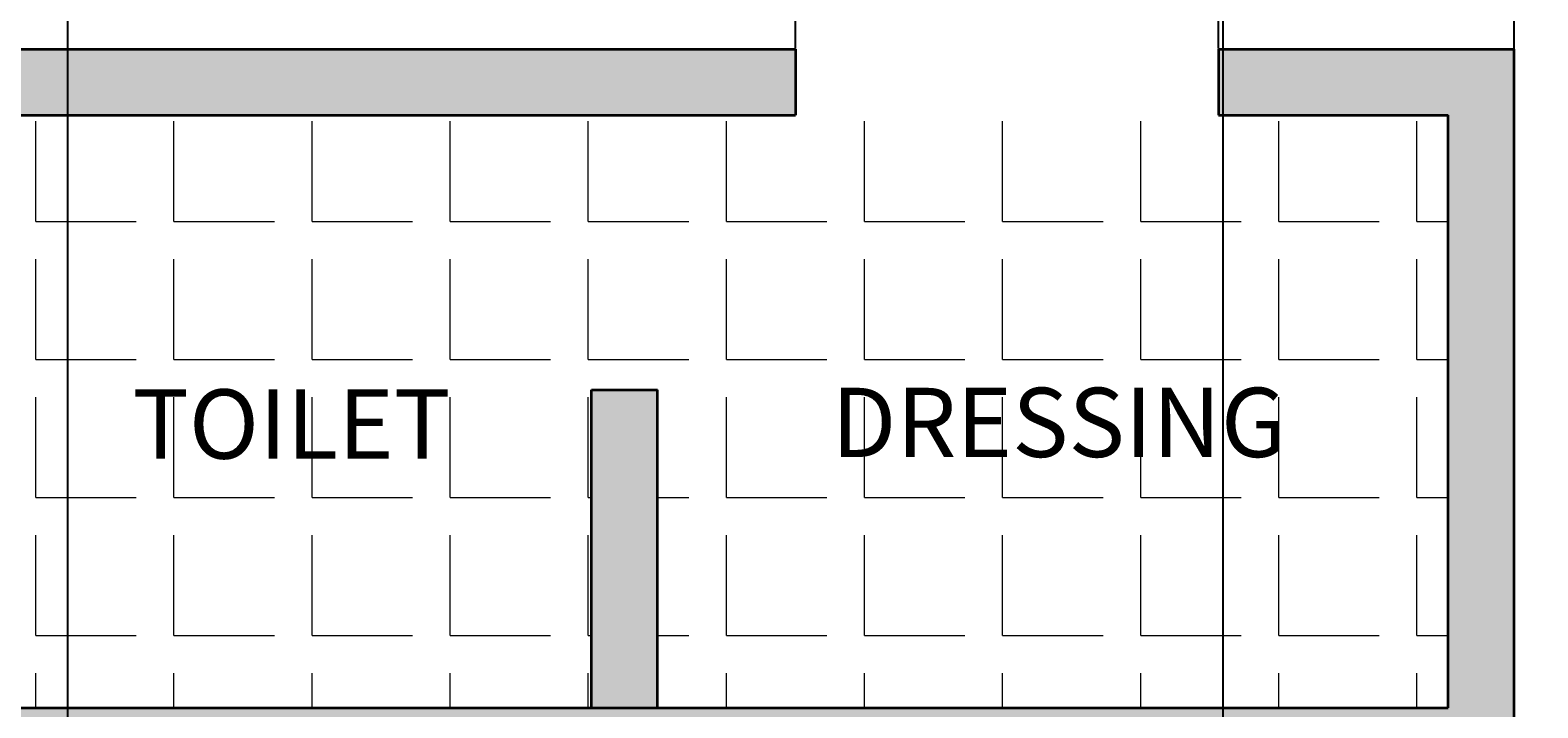
# Model space of a CAD drawing. Units: inches. Extents: x 2549 to 3108, y 1683 to 2362.
# Tile 17 of 30: x 2678 to 2815, y 2081 to 2142. Entities that reach past the tile are written whole.
import ezdxf

# ---------------------------------------------------------------- set-up
doc = ezdxf.new("R2010")
doc.units = ezdxf.units.IN
for name, color, linetype, lineweight in [('A-ANNO-DIMS', 2, 'Continuous', 18), ('A-AREA-IDEN', 7, 'Continuous', 18), ('A-FLOR-PATT', 8, 'Continuous', 13), ('A-FURN-PATT', 9, 'Continuous', 13), ('A-WALL', 7, 'Continuous', 35), ('A-WALL-PATT', 89, 'Continuous', 13)]:
    doc.layers.add(name, color=color, linetype=linetype, lineweight=lineweight)
doc.layers.add('C-PKNG-VEHI-PATT', color=251, linetype='Continuous', lineweight=13, true_color=0x636466)
doc.layers.add('C-PVMT-PATT', color=9, linetype='Continuous', lineweight=13, true_color=0xc7c8ca)
doc.styles.get("Standard").update_dxf_attribs({"font": 'arial.ttf'})
doc.dimstyles.get("Standard").update_dxf_attribs({"dimtxt": 0.18, "dimasz": 0.18, "dimexe": 0.18, "dimexo": 0.0625, "dimgap": 0.09, "dimtad": 0, "dimtih": 1, "dimtoh": 1, "dimdec": 4, "dimzin": 0, "dimdsep": 46, "dimtxsty": 'Standard', "dimcen": 0.09, "dimadec": 0, "dimazin": 0, "dimtfac": 1, "dimtdec": 4, "dimtofl": 0, "dimtmove": 0, "dimatfit": 3, "dimfxl": 1, "dimtolj": 1, "dimtzin": 0, "dimarcsym": 0})

# ---------------------------------------------------------------- blocks, each defined once
blk = doc.blocks.new('*D40')
at = {"layer": 'A-ANNO-DIMS', "color": 0, "lineweight": -2, "transparency": 16777216}
for p, q in [((2747.21, 2140.59), (2747.21, 2171.6)), ((2747.39, 2171.42), (2766, 2171.42)), ((2785.54, 2171.42), (2766.93, 2171.42)), ((2785.72, 2140.59), (2785.72, 2171.6))]:
    blk.add_line(p, q, dxfattribs=at)
at = {"layer": 'A-ANNO-DIMS', "color": 0, "transparency": 16777216}
for points in [[(2747.39, 2171.45), (2747.39, 2171.39), (2747.21, 2171.42)], [(2785.54, 2171.45), (2785.54, 2171.39), (2785.72, 2171.42)]]:
    blk.add_solid(points, dxfattribs=at)
at = {"layer": 'Defpoints', "color": 0, "transparency": 16777216}
for p in [(2785.72, 2171.42), (2747.21, 2140.52), (2785.72, 2140.52)]:
    blk.add_point(p, dxfattribs=at)
at = {"layer": 'A-ANNO-DIMS', "color": 0, "transparency": 16777216, "insert": (2766.47, 2171.42), "char_height": 0.18, "attachment_point": 5}
blk.add_mtext('\\A1;38.505', dxfattribs=at)
blk = doc.blocks.new('*D46')
at = {"layer": 'A-ANNO-DIMS', "color": 0, "lineweight": -2, "transparency": 16777216}
for p, q in [((2812.64, 2140.46), (2812.64, 1683.44)), ((3034.64, 2134.46), (3034.64, 1683.44)), ((2812.82, 1683.62), (2923.35, 1683.62)), ((3034.46, 1683.62), (2923.93, 1683.62))]:
    blk.add_line(p, q, dxfattribs=at)
at = {"layer": 'A-ANNO-DIMS', "color": 0, "transparency": 16777216}
for points in [[(2812.82, 1683.65), (2812.82, 1683.59), (2812.64, 1683.62)], [(3034.46, 1683.65), (3034.46, 1683.59), (3034.64, 1683.62)]]:
    blk.add_solid(points, dxfattribs=at)
at = {"layer": 'Defpoints', "color": 0, "transparency": 16777216}
for p in [(2812.64, 2140.52), (3034.64, 2134.52), (3034.64, 1683.62)]:
    blk.add_point(p, dxfattribs=at)
at = {"layer": 'A-ANNO-DIMS', "color": 0, "transparency": 16777216, "insert": (2923.64, 1683.62), "char_height": 0.18, "attachment_point": 5}
blk.add_mtext('\\A1;222', dxfattribs=at)
blk = doc.blocks.new('*D52')
at = {"layer": 'A-ANNO-DIMS', "color": 0, "lineweight": -2, "transparency": 16777216}
for p, q in [((2812.64, 1891.59), (2812.64, 2362.32)), ((2812.82, 2362.14), (2842.42, 2362.14)), ((2872.46, 2362.14), (2842.86, 2362.14)), ((2872.64, 1891.59), (2872.64, 2362.32))]:
    blk.add_line(p, q, dxfattribs=at)
at = {"layer": 'A-ANNO-DIMS', "color": 0, "transparency": 16777216}
for points in [[(2812.82, 2362.17), (2812.82, 2362.11), (2812.64, 2362.14)], [(2872.46, 2362.17), (2872.46, 2362.11), (2872.64, 2362.14)]]:
    blk.add_solid(points, dxfattribs=at)
at = {"layer": 'Defpoints', "color": 0, "transparency": 16777216}
for p in [(2872.64, 2362.14), (2812.64, 1891.52), (2872.64, 1891.52)]:
    blk.add_point(p, dxfattribs=at)
at = {"layer": 'A-ANNO-DIMS', "color": 0, "transparency": 16777216, "insert": (2842.64, 2362.14), "char_height": 0.18, "attachment_point": 5}
blk.add_mtext('\\A1;60', dxfattribs=at)
blk = doc.blocks.new('*D59')
at = {"layer": 'A-ANNO-DIMS', "color": 0, "lineweight": -2, "transparency": 16777216}
for p, q in [((2680.98, 1761.59), (2680.98, 2362.32)), ((2681.16, 2362.14), (2733.11, 2362.14)), ((2785.98, 2362.14), (2734.02, 2362.14)), ((2786.16, 1761.59), (2786.16, 2362.32))]:
    blk.add_line(p, q, dxfattribs=at)
at = {"layer": 'A-ANNO-DIMS', "color": 0, "transparency": 16777216}
for points in [[(2681.16, 2362.17), (2681.16, 2362.11), (2680.98, 2362.14)], [(2785.98, 2362.17), (2785.98, 2362.11), (2786.16, 2362.14)]]:
    blk.add_solid(points, dxfattribs=at)
at = {"layer": 'Defpoints', "color": 0, "transparency": 16777216}
for p in [(2786.16, 2362.14), (2680.98, 1761.52), (2786.16, 1761.52)]:
    blk.add_point(p, dxfattribs=at)
at = {"layer": 'A-ANNO-DIMS', "color": 0, "transparency": 16777216, "insert": (2733.57, 2362.14), "char_height": 0.18, "attachment_point": 5}
blk.add_mtext('\\A1;105.18', dxfattribs=at)

msp = doc.modelspace()

# ---------------------------------------------------------------- hatches: boundary and pattern name
at = {"layer": 'A-FLOR-PATT', "transparency": 33554567}
h = msp.add_hatch(dxfattribs=at)
h.set_pattern_fill('ANGLE', color=256, scale=1.8)
h.set_pattern_definition([(0, (0, 0), (0, 12.573), [9.144, -3.429]), (90, (0, 0), (-12.573, 8e-16), [9.144, -3.429])])
h.paths.add_polyline_path([(2806.6427, 2134.5237), (2785.7177, 2134.5237), (2747.213, 2134.5237), (2638.6427, 2134.5237), (2638.6427, 2080.5237), (2728.6427, 2080.5237), (2728.6427, 2109.4935), (2734.6427, 2109.4935), (2734.6427, 2080.5237), (2806.6427, 2080.5237)])
h.paths.add_polyline_path([(2673.3659, 2106.0669, -0.50131678), (2654.5049, 2101.1116), (2648.5048, 2103.1116), (2648.5048, 2100.1116), (2650.0048, 2100.1116), (2650.0048, 2097.1116), (2649.0048, 2097.1116), (2649.0048, 2099.1116), (2648.5048, 2099.1116), (2648.5048, 2096.6116), (2640.5048, 2096.6116), (2640.5048, 2117.6116), (2648.5048, 2117.6116), (2648.5048, 2111.1116), (2654.5047, 2113.1116, -0.50132349), (2673.3659, 2108.1563, -0.13289091)], flags=16)
h.paths.add_polyline_path([(2672.0278, 2105.4676, -0.48007965), (2654.5048, 2103.1117), (2654.5048, 2111.1116, -0.4800795), (2672.0278, 2108.7557, -0.21500378)], flags=0)
h.paths.add_polyline_path([(2647.5048, 2115.6116), (2647.5048, 2098.6116, -0.50000012), (2646.5048, 2097.6116), (2642.5048, 2097.6116, -0.50000012), (2641.5048, 2098.6116), (2641.5048, 2115.6116, -0.50000012), (2642.5048, 2116.6116), (2646.5048, 2116.6116, -0.50000012)], flags=0)
h.paths.add_polyline_path([(2748.8496, 2101.6383), (2798.148, 2101.6383), (2798.148, 2111.4248), (2748.8496, 2111.4248)], flags=24)
h.paths.add_polyline_path([(2685.2081, 2101.489), (2719.3253, 2101.489), (2719.3253, 2111.2819), (2685.2081, 2111.2819)], flags=24)
at = {"layer": 'A-FURN-PATT', "transparency": 33554567}
h = msp.add_hatch(color=256, dxfattribs=at)
h.dxf.hatch_style = 1
h.paths.add_polyline_path([(2708.7147, 2271.6737), (2675.2813, 2271.6737), (2675.2813, 2262.0404), (2708.7147, 2262.0404)])
h.paths.add_polyline_path([(2980.8246, 2271.6737), (2947.3913, 2271.6737), (2947.3913, 2262.0404), (2980.8246, 2262.0404)])
h.paths.add_polyline_path([(2748.8496, 2101.6383), (2798.148, 2101.6383), (2798.148, 2111.4248), (2748.8496, 2111.4248)], flags=9)
h.paths.add_polyline_path([(2685.2081, 2101.489), (2719.3253, 2101.489), (2719.3253, 2111.2819), (2685.2081, 2111.2819)], flags=9)
h.paths.add_polyline_path([(2814.6852, 1907.1328), (2847.8384, 1907.1328), (2847.8384, 1916.9258), (2814.6852, 1916.9258)], flags=9)
h.paths.add_polyline_path([(2814.3906, 1835.5864), (2848.0172, 1835.5864), (2848.0172, 1845.3794), (2814.3906, 1845.3794)], flags=9)
h.paths.add_polyline_path([(2800.5245, 1759.1674), (2853.7435, 1759.1674), (2853.7435, 1768.954), (2800.5245, 1768.954)], flags=9)
h.paths.add_polyline_path([(2972.4611, 1807.3305), (3015.3943, 1807.3305), (3015.3943, 1817.117), (2972.4611, 1817.117)], flags=9)
h.paths.add_polyline_path([(2902.3327, 1888.6731), (2937.9131, 1888.6731), (2937.9131, 1898.4661), (2902.3327, 1898.4661)], flags=9)
h.paths.add_polyline_path([(2712.1779, 1878.9039), (2754.1257, 1878.9039), (2754.1257, 1888.6904), (2712.1779, 1888.6904)], flags=9)
h.paths.add_polyline_path([(2614.0056, 2012.812), (2650.0251, 2012.812), (2650.0251, 2022.4371), (2614.0056, 2022.4371)], flags=9)
h.paths.add_polyline_path([(2713.3129, 2003.1645), (2747.4237, 2003.1645), (2747.4237, 2012.951), (2713.3129, 2012.951)], flags=9)
h.paths.add_polyline_path([(2950.1379, 2001.6934), (2982.2992, 2001.6934), (2982.2992, 2011.48), (2950.1379, 2011.48)], flags=9)
h.paths.add_polyline_path([(2940.864, 2238.5537), (2997.5066, 2238.5537), (2997.5066, 2248.3466), (2940.864, 2248.3466)], flags=9)
h.paths.add_polyline_path([(2821.5457, 2202.8348), (2855.663, 2202.8348), (2855.663, 2212.6278), (2821.5457, 2212.6278)], flags=9)
h.paths.add_polyline_path([(2661.8026, 2238.6249), (2718.4451, 2238.6249), (2718.4451, 2248.4179), (2661.8026, 2248.4179)], flags=9)
h = msp.add_hatch(color=256, dxfattribs=at)
h.dxf.hatch_style = 1
h.paths.add_polyline_path([(2906.5064, 1905.2148), (2905.2584, 1904.3827), (2907.0611, 1900.7772), (2908.3092, 1901.6092)])
h.paths.add_polyline_path([(2936.522, 1914.8044), (2935.2739, 1915.6364), (2932.6391, 1912.5856), (2933.8871, 1911.7535)])
h.paths.add_polyline_path([(2950.2508, 1905.6518), (2949.0027, 1906.4839), (2947.1999, 1902.8783), (2948.448, 1902.0463)])
h.paths.add_polyline_path([(2958.5713, 1918.1326), (2956.9072, 1919.242), (2952.4696, 1908.98, 1.38742744), (2954.9657, 1907.3159)])
h.paths.add_polyline_path([(2945.2585, 1927.0078), (2943.5944, 1928.1172), (2934.9965, 1920.6287, 1.38742744), (2937.4927, 1918.9646)])
h.paths.add_polyline_path([(2748.8496, 2101.6383), (2798.148, 2101.6383), (2798.148, 2111.4248), (2748.8496, 2111.4248)], flags=9)
h.paths.add_polyline_path([(2685.2081, 2101.489), (2719.3253, 2101.489), (2719.3253, 2111.2819), (2685.2081, 2111.2819)], flags=9)
h.paths.add_polyline_path([(2814.6852, 1907.1328), (2847.8384, 1907.1328), (2847.8384, 1916.9258), (2814.6852, 1916.9258)], flags=9)
h.paths.add_polyline_path([(2814.3906, 1835.5864), (2848.0172, 1835.5864), (2848.0172, 1845.3794), (2814.3906, 1845.3794)], flags=9)
h.paths.add_polyline_path([(2800.5245, 1759.1674), (2853.7435, 1759.1674), (2853.7435, 1768.954), (2800.5245, 1768.954)], flags=9)
h.paths.add_polyline_path([(2972.4611, 1807.3305), (3015.3943, 1807.3305), (3015.3943, 1817.117), (2972.4611, 1817.117)], flags=9)
h.paths.add_polyline_path([(2902.3327, 1888.6731), (2937.9131, 1888.6731), (2937.9131, 1898.4661), (2902.3327, 1898.4661)], flags=9)
h.paths.add_polyline_path([(2712.1779, 1878.9039), (2754.1257, 1878.9039), (2754.1257, 1888.6904), (2712.1779, 1888.6904)], flags=9)
h.paths.add_polyline_path([(2614.0056, 2012.812), (2650.0251, 2012.812), (2650.0251, 2022.4371), (2614.0056, 2022.4371)], flags=9)
h.paths.add_polyline_path([(2713.3129, 2003.1645), (2747.4237, 2003.1645), (2747.4237, 2012.951), (2713.3129, 2012.951)], flags=9)
h.paths.add_polyline_path([(2950.1379, 2001.6934), (2982.2992, 2001.6934), (2982.2992, 2011.48), (2950.1379, 2011.48)], flags=9)
h.paths.add_polyline_path([(2940.864, 2238.5537), (2997.5066, 2238.5537), (2997.5066, 2248.3466), (2940.864, 2248.3466)], flags=9)
h.paths.add_polyline_path([(2821.5457, 2202.8348), (2855.663, 2202.8348), (2855.663, 2212.6278), (2821.5457, 2212.6278)], flags=9)
h.paths.add_polyline_path([(2661.8026, 2238.6249), (2718.4451, 2238.6249), (2718.4451, 2248.4179), (2661.8026, 2248.4179)], flags=9)
at = {"layer": 'A-WALL-PATT'}
h = msp.add_hatch(color=256, dxfattribs=at)
h.dxf.hatch_style = 1
h.paths.add_polyline_path([(2638.6427, 2272.5237), (3034.6427, 2272.5237), (3034.6427, 1936.5237), (3043.6427, 1936.5237), (3043.6427, 2281.5237), (2629.6427, 2281.5237), (2629.6427, 2074.5237), (2812.6427, 2074.5237), (2812.6427, 2140.5237), (2785.7177, 2140.5237), (2785.7177, 2134.5237), (2806.6427, 2134.5237), (2806.6427, 2080.5237), (2638.6427, 2080.5237)])
h.paths.add_polyline_path([(2638.6427, 1972.5237), (2662.6427, 1972.5237), (2662.6427, 2041.0557), (2653.6427, 2041.0557), (2653.6427, 1978.5237), (2629.6427, 1978.5237), (2629.6427, 1795.5237), (2662.6427, 1795.5237), (2881.6427, 1795.5237), (2881.6427, 1936.5237), (2965.9351, 1936.5237), (2965.9351, 1974.5439), (2959.9351, 1974.5439), (2959.9351, 1945.5237), (2881.6427, 1945.5237), (2872.6427, 1945.5237), (2872.6427, 1804.5237), (2662.6427, 1804.5237), (2638.6427, 1804.5237)])
h = msp.add_hatch(color=256, dxfattribs=at)
h.dxf.hatch_style = 1
h.paths.add_polyline_path([(2747.213, 2140.5237), (2638.6427, 2140.5237), (2638.6427, 2134.5237), (2747.213, 2134.5237)])
h.paths.add_polyline_path([(2734.6427, 2109.4935), (2728.6427, 2109.4935), (2728.6427, 2080.5237), (2734.6427, 2080.5237)])
h.paths.add_polyline_path([(2812.6427, 2074.5237), (2806.6427, 2074.5237), (2806.6427, 2016.1911), (2812.6427, 2016.1911)])
h.paths.add_polyline_path([(2812.6427, 1945.5237), (2806.6427, 1945.5237), (2806.6427, 1885.5237), (2872.6427, 1885.5237), (2872.6427, 1891.5237), (2812.6427, 1891.5237)])
h.paths.add_polyline_path([(2812.6427, 1855.9859), (2806.6427, 1855.9859), (2806.6427, 1804.5237), (2812.6427, 1804.5237)])
at = {"layer": 'C-PKNG-VEHI-PATT'}
h = msp.add_hatch(color=256, dxfattribs=at)
h.dxf.hatch_style = 1
edge = h.paths.add_edge_path()
edge.add_ellipse((2935.7258, 1791.964), major_axis=(-50.66, 0), ratio=0.84230387, start_angle=248.165046, end_angle=265.722579)
edge.add_line((2938.911, 1834.5507), (2925.8653, 1834.5507))
edge.add_ellipse((2929.0505, 1791.964), major_axis=(50.66, 0), ratio=0.84230387, start_angle=94.277421, end_angle=111.834954)
edge.add_line((2912.8508, 1832.3947), (2914.2044, 1822.2495))
edge.add_ellipse((2930.6538, 1783.1023), major_axis=(-49.3014, 0), ratio=0.84230387, start_angle=-85.12993, end_angle=-67.208085, ccw=False)
edge.add_line((2927.1247, 1824.5225), (2937.6516, 1824.5225))
edge.add_ellipse((2934.1225, 1783.1023), major_axis=(49.3014, 0), ratio=0.84230387, start_angle=67.208085, end_angle=85.12993, ccw=False)
edge.add_line((2950.5719, 1822.2495), (2951.9255, 1832.3947))
edge = h.paths.add_edge_path()
edge.add_ellipse((2903.4793, 1857.3351), major_axis=(-34.7979, 0), ratio=0.84230387, start_angle=180, end_angle=209.43857)
edge.add_ellipse((2961.297, 1857.3351), major_axis=(34.7979, 0), ratio=0.84230387, start_angle=150.56143, end_angle=180)
edge.add_line((2926.4991, 1857.3351), (2926.4991, 1843.7609))
edge.add_ellipse((2924.1251, 1844.3143), major_axis=(-0.2209, 3.9278), ratio=0.60383358, start_angle=89.002014, end_angle=253.657408, ccw=False)
edge.add_line((2921.7512, 1844.2222), (2921.7512, 1853.3975))
edge.add_line((2921.7512, 1853.3975), (2925.269, 1855.8484))
edge.add_ellipse((2925.4782, 1855.4931), major_axis=(0.4584, 0), ratio=0.84230387, start_angle=90, end_angle=134.480211, ccw=False)
edge.add_line((2925.4782, 1855.8792), (2926.4991, 1855.8792))
edge.add_line((2926.4991, 1855.8792), (2926.4991, 1857.3351))
edge.add_ellipse((2961.297, 1857.3351), major_axis=(34.7979, 0), ratio=0.84230387, start_angle=150.56143, end_angle=180, ccw=False)
edge.add_line((2932.3882, 1873.6501), (2932.3882, 1875.7801))
edge.add_ellipse((2932.3882, 1875.3939), major_axis=(0.4584, 0), ratio=0.84230387, start_angle=90, end_angle=127.93313)
edge.add_line((2932.1366, 1875.7167), (2928.5915, 1873.7564))
edge.add_ellipse((2899.9271, 2002.4692), major_axis=(155.4756, 0), ratio=0.84230387, start_angle=-80.743434, end_angle=-77.445067, ccw=False)
edge.add_ellipse((2949.4402, 1715.2151), major_axis=(-189.1422, 0), ratio=0.84230387, start_angle=-79.790461, end_angle=-77.555373)
edge.add_ellipse((3300.3614, 1852.5642), major_axis=(-386.1662, 0), ratio=0.84230387, start_angle=-2.863715, end_angle=2.198541)
edge.add_ellipse((2929.0505, 1792.5159), major_axis=(-55.6192, 0), ratio=0.84230387, start_angle=-85.917589, end_angle=-72.280047, ccw=False)
edge.add_line((2925.7129, 1839.2798), (2939.0634, 1839.2798))
edge.add_ellipse((2935.7258, 1792.5159), major_axis=(55.6192, 0), ratio=0.84230387, start_angle=72.280047, end_angle=85.917589, ccw=False)
edge.add_ellipse((2564.4149, 1852.5642), major_axis=(-386.1662, 0), ratio=0.84230387, start_angle=177.801459, end_angle=182.863715)
edge.add_ellipse((2915.3361, 1715.2151), major_axis=(189.1422, 0), ratio=0.84230387, start_angle=77.555373, end_angle=79.790461)
edge.add_ellipse((2964.8492, 2002.4692), major_axis=(-155.4756, 0), ratio=0.84230387, start_angle=77.445067, end_angle=80.743434, ccw=False)
edge.add_line((2936.1848, 1873.7564), (2932.6397, 1875.7167))
edge.add_ellipse((2932.3882, 1875.3939), major_axis=(0.4584, 0), ratio=0.84230387, start_angle=52.06687, end_angle=90)
edge.add_line((2932.3882, 1875.7801), (2932.3882, 1873.6501))
edge.add_ellipse((2903.4793, 1857.3351), major_axis=(-34.7979, 0), ratio=0.84230387, start_angle=180, end_angle=209.43857, ccw=False)
edge.add_line((2938.2772, 1857.3351), (2938.2772, 1855.8792))
edge.add_line((2938.2772, 1855.8792), (2939.4059, 1855.8792))
edge.add_ellipse((2939.2981, 1855.4931), major_axis=(-0.4584, 0), ratio=0.84230387, start_angle=225.519789, end_angle=270, ccw=False)
edge.add_line((2939.5903, 1855.7906), (2943.0251, 1853.3975))
edge.add_line((2943.0251, 1853.3975), (2943.0251, 1844.2222))
edge.add_ellipse((2940.6512, 1844.3143), major_axis=(0.2209, 3.9278), ratio=0.60383358, start_angle=106.342592, end_angle=270.997986, ccw=False)
edge.add_line((2938.2772, 1843.7609), (2938.2772, 1857.3351))
edge = h.paths.add_edge_path()
edge.add_ellipse((2932.3882, 1865.1973), major_axis=(91.081, 0), ratio=0.84230387, start_angle=256.401865, end_angle=283.598135, ccw=False)
edge.add_line((2914.2044, 1790.0239), (2914.2044, 1778.3622))
edge.add_ellipse((2932.3882, 1853.5356), major_axis=(91.081, 0), ratio=0.84230387, start_angle=256.401865, end_angle=283.598135)
edge.add_line((2950.5719, 1778.3622), (2950.5719, 1790.0239))
edge = h.paths.add_edge_path()
edge.add_ellipse((2948.7383, 1772.3145), major_axis=(1.8336, 0), ratio=0.84230387, start_angle=0, end_angle=90)
edge.add_line((2948.7383, 1773.859), (2916.038, 1773.859))
edge.add_ellipse((2916.038, 1772.3145), major_axis=(1.8336, 0), ratio=0.84230387, start_angle=90, end_angle=180)
edge.add_line((2914.2044, 1772.3145), (2914.2044, 1760.2558))
edge.add_line((2914.2044, 1760.2558), (2950.5719, 1760.2558))
edge.add_line((2950.5719, 1760.2558), (2950.5719, 1772.3145))
h.paths.add_polyline_path([(2748.8496, 2101.6383), (2798.148, 2101.6383), (2798.148, 2111.4248), (2748.8496, 2111.4248)], flags=9)
h.paths.add_polyline_path([(2685.2081, 2101.489), (2719.3253, 2101.489), (2719.3253, 2111.2819), (2685.2081, 2111.2819)], flags=9)
h.paths.add_polyline_path([(2814.6852, 1907.1328), (2847.8384, 1907.1328), (2847.8384, 1916.9258), (2814.6852, 1916.9258)], flags=9)
h.paths.add_polyline_path([(2814.3906, 1835.5864), (2848.0172, 1835.5864), (2848.0172, 1845.3794), (2814.3906, 1845.3794)], flags=9)
h.paths.add_polyline_path([(2800.5245, 1759.1674), (2853.7435, 1759.1674), (2853.7435, 1768.954), (2800.5245, 1768.954)], flags=9)
h.paths.add_polyline_path([(2972.4611, 1807.3305), (3015.3943, 1807.3305), (3015.3943, 1817.117), (2972.4611, 1817.117)], flags=9)
h.paths.add_polyline_path([(2902.3327, 1888.6731), (2937.9131, 1888.6731), (2937.9131, 1898.4661), (2902.3327, 1898.4661)], flags=9)
h.paths.add_polyline_path([(2712.1779, 1878.9039), (2754.1257, 1878.9039), (2754.1257, 1888.6904), (2712.1779, 1888.6904)], flags=9)
h.paths.add_polyline_path([(2614.0056, 2012.812), (2650.0251, 2012.812), (2650.0251, 2022.4371), (2614.0056, 2022.4371)], flags=9)
h.paths.add_polyline_path([(2713.3129, 2003.1645), (2747.4237, 2003.1645), (2747.4237, 2012.951), (2713.3129, 2012.951)], flags=9)
h.paths.add_polyline_path([(2950.1379, 2001.6934), (2982.2992, 2001.6934), (2982.2992, 2011.48), (2950.1379, 2011.48)], flags=9)
h.paths.add_polyline_path([(2940.864, 2238.5537), (2997.5066, 2238.5537), (2997.5066, 2248.3466), (2940.864, 2248.3466)], flags=9)
h.paths.add_polyline_path([(2821.5457, 2202.8348), (2855.663, 2202.8348), (2855.663, 2212.6278), (2821.5457, 2212.6278)], flags=9)
h.paths.add_polyline_path([(2661.8026, 2238.6249), (2718.4451, 2238.6249), (2718.4451, 2248.4179), (2661.8026, 2248.4179)], flags=9)
at = {"layer": 'C-PVMT-PATT'}
h = msp.add_hatch(color=256, dxfattribs=at)
h.dxf.hatch_style = 1
h.paths.add_polyline_path([(3067.6427, 2305.5237), (2605.6427, 2305.5237), (2605.6427, 2074.5237), (2629.6427, 2074.5237), (2629.6427, 2281.5237), (3043.6427, 2281.5237), (3043.6427, 1885.5237), (3043.6427, 1872.8745), (3031.1672, 1872.8745), (3031.1672, 1862.5731), (2995.8054, 1862.5731), (2995.8054, 1872.8745), (2983.1752, 1872.8745), (2983.1752, 1885.5237), (2881.6427, 1885.5237), (2881.6427, 1795.5237), (2751.0977, 1795.5237), (2751.0977, 1761.5237), (2786.1577, 1761.5237), (2786.1577, 1723.5237), (2881.84, 1723.5237), (2881.84, 1714.5237), (3067.6427, 1714.5237), (3067.6427, 1723.5237)])
edge = h.paths.add_edge_path(flags=16)
edge.add_ellipse((2949.4402, 1710.9683), major_axis=(-194.1014, 0), ratio=0.84230387, start_angle=-77.874034, end_angle=-76.219471, ccw=False)
edge.add_ellipse((2949.4402, 1715.2151), major_axis=(-189.1422, 0), ratio=0.84230387, start_angle=-79.790461, end_angle=-77.555373, ccw=False)
edge.add_ellipse((2899.9271, 2002.4692), major_axis=(155.4756, 0), ratio=0.84230387, start_angle=-80.743434, end_angle=-77.445067)
edge.add_line((2928.5915, 1873.7564), (2932.3882, 1875.8558))
edge.add_line((2932.3882, 1875.8558), (2936.1848, 1873.7564))
edge.add_ellipse((2964.8492, 2002.4692), major_axis=(-155.4756, 0), ratio=0.84230387, start_angle=77.445067, end_angle=80.743434)
edge.add_ellipse((2915.3361, 1715.2151), major_axis=(189.1422, 0), ratio=0.84230387, start_angle=77.555373, end_angle=79.790461, ccw=False)
edge.add_ellipse((2915.3361, 1710.9683), major_axis=(-194.1014, 0), ratio=0.84230387, start_angle=256.219471, end_angle=257.874034, ccw=False)
edge.add_ellipse((2628.2871, 1850.2612), major_axis=(-327.2532, 0), ratio=0.84230387, start_angle=182.17995, end_angle=183.650428, ccw=False)
edge.add_ellipse((2955.5637, 1861.9334), major_axis=(-0.9168, 0), ratio=0.84230387, start_angle=180, end_angle=270, ccw=False)
edge.add_line((2956.4805, 1862.3857), (2956.4805, 1846.4866))
edge.add_ellipse((2955.5637, 1846.939), major_axis=(-0.9168, 0), ratio=0.84230387, start_angle=90, end_angle=180, ccw=False)
edge.add_ellipse((-3607.0606, 1835.832), major_axis=(-6562.6242, 0), ratio=0.84230387, start_angle=179.61613322, end_angle=180.09022909, ccw=False)
edge.add_ellipse((2955.5637, 1791.0926), major_axis=(0.9168, 0), ratio=0.84230387, start_angle=0, end_angle=90, ccw=False)
edge.add_line((2956.4805, 1791.545), (2956.4805, 1775.6459))
edge.add_ellipse((2955.5637, 1776.0982), major_axis=(0.9168, 0), ratio=0.84230387, start_angle=270, end_angle=360, ccw=False)
edge.add_ellipse((-3607.0606, 1835.832), major_axis=(-6562.6242, 0), ratio=0.84230387, start_angle=179.3813568, end_angle=179.47172853, ccw=False)
edge.add_ellipse((2954.5907, 1763.8768), major_axis=(-1.3752, 0), ratio=0.84230387, start_angle=179.371763, end_angle=248.464757, ccw=False)
edge.add_ellipse((-3607.519, 1835.832), major_axis=(-6564.0409, 0), ratio=0.842303863, start_angle=179.35344594, end_angle=179.37176282, ccw=False)
edge.add_ellipse((2952.6829, 1761.8002), major_axis=(3.2503, 0), ratio=0.84230387, start_angle=-90, end_angle=-0.646554, ccw=False)
edge.add_line((2952.6829, 1759.0625), (2912.0934, 1759.0625))
edge.add_ellipse((2912.0934, 1761.8002), major_axis=(3.2503, 0), ratio=0.84230387, start_angle=180.646554, end_angle=270, ccw=False)
edge.add_ellipse((9472.2953, 1835.832), major_axis=(-6564.0409, 0), ratio=0.842303871, start_angle=0.62823722, end_angle=0.6465541, ccw=False)
edge.add_ellipse((2910.1856, 1763.8768), major_axis=(1.3752, 0), ratio=0.84230387, start_angle=111.535244, end_angle=180.628237, ccw=False)
edge.add_ellipse((9471.8369, 1835.832), major_axis=(-6562.6242, 0), ratio=0.84230387, start_angle=0.52827147, end_angle=0.6465541, ccw=False)
edge.add_ellipse((2909.2126, 1776.0982), major_axis=(-0.9168, 0), ratio=0.84230387, start_angle=0, end_angle=90, ccw=False)
edge.add_line((2908.2958, 1775.6459), (2908.2958, 1791.545))
edge.add_ellipse((2909.2126, 1791.0926), major_axis=(-0.9168, 0), ratio=0.84230387, start_angle=-90, end_angle=0, ccw=False)
edge.add_ellipse((9471.8369, 1835.832), major_axis=(-6562.6242, 0), ratio=0.84230387, start_angle=-0.09022909, end_angle=0.38386678, ccw=False)
edge.add_ellipse((2909.2126, 1846.939), major_axis=(-0.9168, 0), ratio=0.84230387, start_angle=0, end_angle=90, ccw=False)
edge.add_line((2908.2958, 1846.4866), (2908.2958, 1862.3857))
edge.add_ellipse((2909.2126, 1861.9334), major_axis=(0.9168, 0), ratio=0.84230387, start_angle=90, end_angle=180, ccw=False)
edge.add_ellipse((3236.4892, 1850.2612), major_axis=(327.2532, 0), ratio=0.84230387, start_angle=176.349572, end_angle=177.82005, ccw=False)
edge = h.paths.add_edge_path(flags=0)
edge.add_ellipse((2903.4793, 1857.3351), major_axis=(-34.7979, 0), ratio=0.84230387, start_angle=180, end_angle=209.43857, ccw=False)
edge.add_line((2938.2772, 1857.3351), (2938.2772, 1855.8792))
edge.add_line((2938.2772, 1855.8792), (2939.4631, 1855.8792))
edge.add_line((2939.4631, 1855.8792), (2943.0251, 1853.3975))
edge.add_line((2943.0251, 1853.3975), (2943.0251, 1844.2222))
edge.add_ellipse((2940.6512, 1844.3143), major_axis=(0.2209, 3.9278), ratio=0.60383358, start_angle=106.342592, end_angle=270.997986, ccw=False)
edge.add_line((2938.2772, 1843.7609), (2938.2772, 1857.3351))
edge.add_ellipse((2903.4793, 1857.3351), major_axis=(-34.7979, 0), ratio=0.84230387, start_angle=180, end_angle=209.43857)
edge.add_ellipse((2961.297, 1857.3351), major_axis=(34.7979, 0), ratio=0.84230387, start_angle=150.56143, end_angle=180)
edge.add_line((2926.4991, 1857.3351), (2926.4991, 1843.7609))
edge.add_ellipse((2924.1251, 1844.3143), major_axis=(-0.2209, 3.9278), ratio=0.60383358, start_angle=89.002014, end_angle=253.657408, ccw=False)
edge.add_line((2921.7512, 1844.2222), (2921.7512, 1853.3975))
edge.add_line((2921.7512, 1853.3975), (2925.3132, 1855.8792))
edge.add_line((2925.3132, 1855.8792), (2926.4991, 1855.8792))
edge.add_line((2926.4991, 1855.8792), (2926.4991, 1857.3351))
edge.add_ellipse((2961.297, 1857.3351), major_axis=(34.7979, 0), ratio=0.84230387, start_angle=150.56143, end_angle=180, ccw=False)
edge = h.paths.add_edge_path(flags=0)
edge.add_ellipse((2929.0505, 1791.964), major_axis=(50.66, 0), ratio=0.84230387, start_angle=94.277421, end_angle=111.834954, ccw=False)
edge.add_line((2925.8653, 1834.5507), (2938.911, 1834.5507))
edge.add_ellipse((2935.7258, 1791.964), major_axis=(-50.66, 0), ratio=0.84230387, start_angle=248.165046, end_angle=265.722579, ccw=False)
edge.add_line((2951.9255, 1832.3947), (2950.5719, 1822.2495))
edge.add_ellipse((2934.1225, 1783.1023), major_axis=(49.3014, 0), ratio=0.84230387, start_angle=67.208085, end_angle=85.12993)
edge.add_line((2937.6516, 1824.5225), (2927.1247, 1824.5225))
edge.add_ellipse((2930.6538, 1783.1023), major_axis=(-49.3014, 0), ratio=0.84230387, start_angle=-85.12993, end_angle=-67.208085)
edge.add_line((2914.2044, 1822.2495), (2912.8508, 1832.3947))
edge = h.paths.add_edge_path(flags=0)
edge.add_line((2910.1338, 1829.4651), (2912.6432, 1821.2711))
edge.add_ellipse((5203.7787, 1816.4367), major_axis=(-2291.1426, 0), ratio=0.84230387, start_angle=-0.1208974, end_angle=0.3640763)
edge.add_line((2912.7012, 1801.8782), (2910.3305, 1792.5698))
edge.add_ellipse((9471.8369, 1835.832), major_axis=(-6561.7074, 0), ratio=0.84230387, start_angle=0.05559431, end_angle=0.37776419, ccw=False)
edge = h.paths.add_edge_path(flags=0)
edge.add_ellipse((-3607.0606, 1835.832), major_axis=(6561.7074, 0), ratio=0.84230387, start_angle=-0.37776419, end_angle=-0.05559431, ccw=False)
edge.add_line((2954.4458, 1792.5698), (2952.0751, 1801.8782))
edge.add_ellipse((660.9976, 1816.4367), major_axis=(2291.1426, 0), ratio=0.84230387, start_angle=-0.3640763, end_angle=0.1208974)
edge.add_line((2952.1331, 1821.2711), (2954.6425, 1829.4651))
edge = h.paths.add_edge_path(flags=0)
edge.add_ellipse((2932.3882, 1865.1973), major_axis=(91.081, 0), ratio=0.84230387, start_angle=256.401865, end_angle=283.598135)
edge.add_line((2950.5719, 1790.0239), (2950.5719, 1778.3622))
edge.add_ellipse((2932.3882, 1853.5356), major_axis=(91.081, 0), ratio=0.84230387, start_angle=256.401865, end_angle=283.598135, ccw=False)
edge.add_line((2914.2044, 1778.3622), (2914.2044, 1790.0239))
edge = h.paths.add_edge_path(flags=0)
edge.add_line((2916.038, 1773.859), (2948.7383, 1773.859))
edge.add_ellipse((2948.7383, 1772.3145), major_axis=(1.8336, 0), ratio=0.84230387, start_angle=0, end_angle=90, ccw=False)
edge.add_line((2950.5719, 1772.3145), (2950.5719, 1760.2558))
edge.add_line((2950.5719, 1760.2558), (2914.2044, 1760.2558))
edge.add_line((2914.2044, 1760.2558), (2914.2044, 1772.3145))
edge.add_ellipse((2916.038, 1772.3145), major_axis=(1.8336, 0), ratio=0.84230387, start_angle=90, end_angle=180, ccw=False)
h.paths.add_polyline_path([(2629.6427, 1978.5237), (2605.6427, 1978.5237), (2605.6427, 1723.5237), (2629.6427, 1723.5237), (2629.6427, 1795.5237)], flags=17)
h.paths.add_polyline_path([(2800.5245, 1759.1674), (2853.7435, 1759.1674), (2853.7435, 1768.954), (2800.5245, 1768.954)], flags=24)
h.paths.add_polyline_path([(2972.4611, 1807.3305), (3015.3943, 1807.3305), (3015.3943, 1817.117), (2972.4611, 1817.117)], flags=24)

# ---------------------------------------------------------------- linework, layer by layer
at = {"layer": 'A-WALL'}
for p, q in [((2638.6427, 2140.5237), (2747.213, 2140.5237)), ((2747.213, 2140.5237), (2747.213, 2134.5237)), ((2785.7177, 2140.5237), (2785.7177, 2134.5237)), ((2785.7177, 2140.5237), (2812.6427, 2140.5237)), ((2812.6427, 2074.5237), (2812.6427, 2140.5237)), ((2638.6427, 2134.5237), (2747.213, 2134.5237)), ((2785.7177, 2134.5237), (2806.6427, 2134.5237)), ((2806.6427, 2080.5237), (2806.6427, 2134.5237)), ((2728.6427, 2080.5237), (2728.6427, 2109.4935)), ((2728.6427, 2109.4935), (2734.6427, 2109.4935)), ((2734.6427, 2080.5237), (2734.6427, 2109.4935)), ((2638.6427, 2080.5237), (2806.6427, 2080.5237))]:
    msp.add_line(p, q, dxfattribs=at)

# ---------------------------------------------------------------- texts
at = {"layer": 'A-AREA-IDEN'}
for s, p in [('TOILET', (2686.8402, 2103.2287)), ('DRESSING', (2750.4807, 2103.377))]:
    msp.add_text(s, height=6.30916, dxfattribs=at).set_placement(p)

# ---------------------------------------------------------------- dimensions: what is measured, and where the dimension line sits
at = {"layer": 'A-ANNO-DIMS'}
for base, p1, p2, override, picture, middle in [((2786.1577, 2362.1425), (2680.9778, 1761.5237), (2786.1577, 1761.5237), {"dimdec": 2, "dimlfac": 1, "dimrnd": 0, "dimzin": 0, "dimdsep": 46, "dimlunit": 2}, '*D59', (2733.5678, 2362.1425)), ((2872.6427, 2362.1425), (2812.6427, 1891.5237), (2872.6427, 1891.5237), {"dimdec": 0, "dimlfac": 1, "dimrnd": 0, "dimzin": 0, "dimdsep": 46, "dimlunit": 2}, '*D52', (2842.6427, 2362.1425)), ((2785.7177, 2171.4237), (2747.213, 2140.5237), (2785.7177, 2140.5237), {"dimdec": 3, "dimlfac": 1, "dimrnd": 0, "dimzin": 0, "dimdsep": 46, "dimlunit": 2}, '*D40', (2766.4653, 2171.4237)), ((3034.6427, 1683.6237), (2812.6427, 2140.5237), (3034.6427, 2134.5237), {"dimdec": 0, "dimlfac": 1, "dimrnd": 0, "dimzin": 0, "dimdsep": 46, "dimlunit": 2}, '*D46', (2923.6427, 1683.6237))]:
    dim = msp.add_linear_dim(base=base, p1=p1, p2=p2, dimstyle='Standard', override=override, dxfattribs=at)
    dim.commit()
    dim.dimension.update_dxf_attribs({"geometry": picture, "text_midpoint": middle})

doc.saveas('drawing.dxf')
